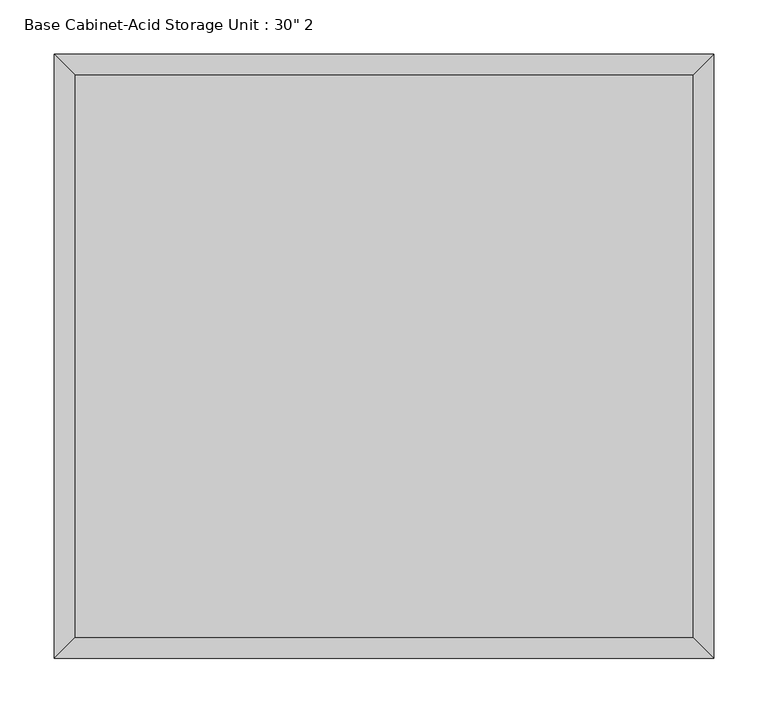
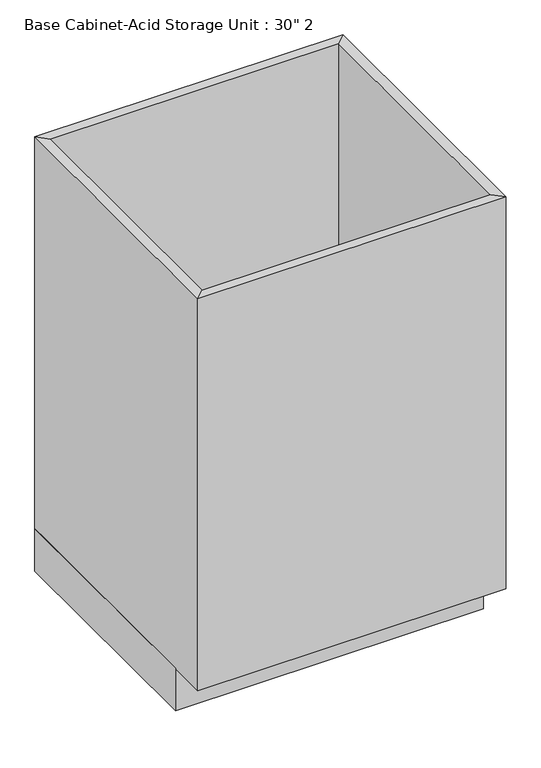
"""IFC4 building model written with IfcOpenShell, lengths in millimetres: furniture geometry."""

from ifc_helpers import new_model, si_unit, frame, origin, origin_with_axes, place, context, project, spatial, polyline, outline, extrude, faceted_brep, source, transform, mapped, element, save


def furniture_6369f5ad(model_context):
    return source(origin(), model_context, "Body", "SolidModel", [
        extrude(outline(polyline([(323.5377049, 0.0), (323.5377049, -482.6), (-286.0622951, -482.6), (-286.0622951, 0.0), (323.5377049, 0.0)])), origin_with_axes(), (0.0, 0.0, 1.0), 88.9),
        faceted_brep([(304.4877049, -539.75, 908.05), (304.4877049, -539.75, 88.9), (-267.0122951, -539.75, 88.9), (-267.0122951, -539.75, 908.05), (323.5377049, -558.8, 908.05), (-286.0622951, -558.8, 908.05), (323.5377049, -558.8, 88.9), (-286.0622951, -558.8, 88.9), (-267.0122951, -19.05, 88.9), (-267.0122951, -19.05, 908.05), (-286.0622951, 0.0, 908.05), (-286.0622951, 0.0, 88.9), (304.4877049, -19.05, 88.9), (304.4877049, -19.05, 908.05), (323.5377049, 0.0, 908.05), (323.5377049, 0.0, 88.9)], [[[0, 1, 2, 3]], [[4, 0, 3, 5]], [[6, 4, 5, 7]], [[1, 6, 7, 2]], [[3, 2, 8, 9]], [[5, 3, 9, 10]], [[7, 5, 10, 11]], [[2, 7, 11, 8]], [[9, 8, 12, 13]], [[10, 9, 13, 14]], [[11, 10, 14, 15]], [[8, 11, 15, 12]], [[13, 12, 1, 0]], [[14, 13, 0, 4]], [[15, 14, 4, 6]], [[12, 15, 6, 1]]]),
        extrude(outline(polyline([(304.4877049, -19.05), (304.4877049, -539.75), (-267.0122951, -539.75), (-267.0122951, -19.05), (304.4877049, -19.05)])), frame((0.0, 0.0, 88.9), z_axis=(0.0, 0.0, 1.0), x_axis=(1.0, 0.0, 0.0)), (0.0, 0.0, 1.0), 19.05),
    ])


if __name__ == "__main__":
    model = new_model("IFC4")
    model_context = context("Model", 3, world=origin())
    ifc_project = project(units=[si_unit("LENGTHUNIT", "METRE", prefix="MILLI")], contexts=[model_context])
    site = spatial("IfcSite", under=ifc_project)
    building = spatial("IfcBuilding", under=site)
    placement = place(None, origin())
    furniture_shape = furniture_6369f5ad(model_context)
    element("IfcFurniture", 1, ObjectType="Base Cabinet-Acid Storage Unit : 30\" 2", at=placement, inside=building, context=model_context, shape_type="MappedRepresentation", body=[
        mapped(furniture_shape, transform((0.0, 0.0, 0.0), x_axis=(1.0, 0.0, 0.0), y_axis=(0.0, 1.0, 0.0), z_axis=(0.0, 0.0, 1.0))),
    ])
    save(model, "model.ifc")

# Revit data of these elements
# Type "Base Cabinet-Acid Storage Unit : 30\" 2"
#   Depth = 1' - 10"
#   Height = 2' - 11 3/4"
#   Toe Depth = 0' - 3"
#   Toe Height = 0' - 3 1/2"
#   Width = 2' - 0"
#   Default Elevation = 0
# Element 1 (IfcFurniture, "Base Cabinet-Acid Storage Unit : 30\" 2")
#   Materials on its faces: "Cabinet"
# Materials
#   "Cabinet": colour RGB 204 122 2, transparency 0
